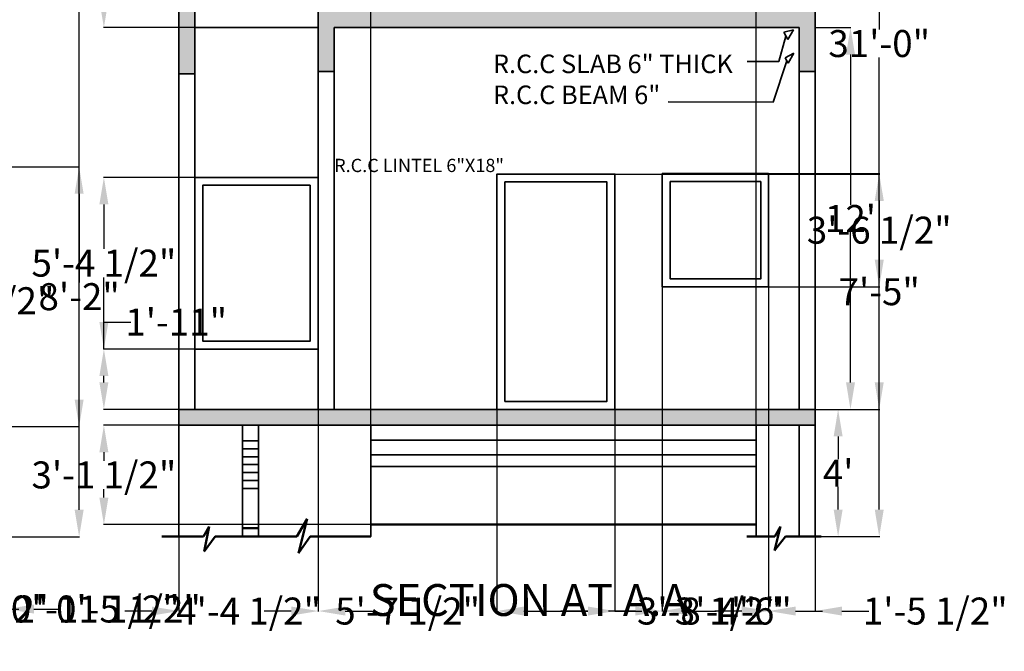
# Model space of a CAD drawing. Units: inches. Extents: x 21 to 3450, y 4 to 2137.
# Tile 7 of 14: x 2431 to 2802, y 1551 to 1790. Entities that reach past the tile are written whole.
import ezdxf

# ---------------------------------------------------------------- set-up
doc = ezdxf.new("R2010")
doc.units = ezdxf.units.IN
doc.header["$MEASUREMENT"] = 0
for name, color, linetype, lineweight in [('A-ANNO-DIMS', 2, 'Continuous', 18), ('A-ANNO-TEXT', 7, 'Continuous', 18), ('A-SECT', 7, 'Continuous', 35), ('A-SECT-PATT', 8, 'Continuous', 13), ('A-WALL', 7, 'Continuous', 50)]:
    doc.layers.add(name, color=color, linetype=linetype, lineweight=lineweight)
doc.styles.get("Standard").update_dxf_attribs({"font": 'arial.ttf'})
doc.dimstyles.get("Standard").update_dxf_attribs({"dimtxt": 10.18, "dimasz": 10.18, "dimexe": 0.18, "dimexo": 0.0625, "dimgap": 0.09, "dimtad": 0, "dimtih": 1, "dimtoh": 1, "dimdec": 0, "dimzin": 0, "dimdsep": 46, "dimlunit": 3, "dimtxsty": 'Standard', "dimcen": 0.09, "dimadec": 0, "dimazin": 0, "dimtfac": 1, "dimtdec": 0, "dimtofl": 0, "dimtmove": 0, "dimatfit": 3, "dimfxl": 1, "dimtolj": 1, "dimtzin": 0, "dimarcsym": 0})

# ---------------------------------------------------------------- blocks, each defined once
blk = doc.blocks.new('*D12')
at = {"layer": 'A-ANNO-DIMS', "color": 0, "lineweight": -2, "transparency": 16777216}
for p, q in [((2731.13, 1642.57), (2739.97, 1642.57)), ((2739.79, 1632.39), (2739.79, 1623.75)), ((2739.79, 1604.75), (2739.79, 1613.39)), ((2731.13, 1594.57), (2739.97, 1594.57))]:
    blk.add_line(p, q, dxfattribs=at)
at = {"layer": 'A-ANNO-DIMS', "color": 0, "transparency": 16777216}
for points in [[(2738.1, 1632.39), (2741.49, 1632.39), (2739.79, 1642.57)], [(2738.1, 1604.75), (2741.49, 1604.75), (2739.79, 1594.57)]]:
    blk.add_solid(points, dxfattribs=at)
at = {"layer": 'Defpoints', "color": 0, "transparency": 16777216}
for p in [(2731.07, 1642.57), (2739.79, 1642.57), (2731.07, 1594.57)]:
    blk.add_point(p, dxfattribs=at)
at = {"layer": 'A-ANNO-DIMS', "color": 0, "transparency": 16777216, "insert": (2739.79, 1618.57), "char_height": 10.18, "attachment_point": 5}
blk.add_mtext("\\A1;4'", dxfattribs=at)
blk = doc.blocks.new('*D13')
at = {"layer": 'A-ANNO-DIMS', "color": 0, "lineweight": -2, "transparency": 16777216}
for p, q in [((2731.13, 1786.57), (2744.63, 1786.57)), ((2744.45, 1776.39), (2744.45, 1719.77)), ((2744.45, 1652.75), (2744.45, 1709.37)), ((2731.19, 1642.57), (2744.63, 1642.57))]:
    blk.add_line(p, q, dxfattribs=at)
at = {"layer": 'A-ANNO-DIMS', "color": 0, "transparency": 16777216}
for points in [[(2742.76, 1776.39), (2746.15, 1776.39), (2744.45, 1786.57)], [(2742.76, 1652.75), (2746.15, 1652.75), (2744.45, 1642.57)]]:
    blk.add_solid(points, dxfattribs=at)
at = {"layer": 'Defpoints', "color": 0, "transparency": 16777216}
for p in [(2731.07, 1786.57), (2744.45, 1786.57), (2731.13, 1642.57)]:
    blk.add_point(p, dxfattribs=at)
at = {"layer": 'A-ANNO-DIMS', "color": 0, "transparency": 16777216, "insert": (2744.45, 1714.57), "char_height": 10.18, "attachment_point": 5}
blk.add_mtext("\\A1;12'", dxfattribs=at)
blk = doc.blocks.new('*D152')
at = {"layer": 'A-ANNO-DIMS', "color": 0, "lineweight": -2, "transparency": 16777216}
for p, q in [((2426.25, 2094.9), (2453.61, 2094.9)), ((2453.43, 2084.72), (2453.43, 1850.06)), ((2453.43, 1604.7), (2453.43, 1839.36)), ((2426.25, 1594.52), (2453.61, 1594.52))]:
    blk.add_line(p, q, dxfattribs=at)
at = {"layer": 'A-ANNO-DIMS', "color": 0, "transparency": 16777216}
for points in [[(2451.74, 2084.72), (2455.13, 2084.72), (2453.43, 2094.9)], [(2451.74, 1604.7), (2455.13, 1604.7), (2453.43, 1594.52)]]:
    blk.add_solid(points, dxfattribs=at)
at = {"layer": 'Defpoints', "color": 0, "transparency": 16777216}
for p in [(2426.18, 2094.9), (2453.43, 2094.9), (2426.18, 1594.52)]:
    blk.add_point(p, dxfattribs=at)
at = {"layer": 'A-ANNO-DIMS', "color": 0, "transparency": 16777216, "insert": (2453.43, 1844.71), "char_height": 10.18, "attachment_point": 5}
blk.add_mtext('\\A1;41\'-8 1/2"', dxfattribs=at)
blk = doc.blocks.new('*D165')
at = {"layer": 'A-ANNO-DIMS', "color": 0, "lineweight": -2, "transparency": 16777216}
for p, q in [((2374.7, 1636.02), (2374.7, 1567.09)), ((2384.8, 1636.02), (2384.8, 1567.09)), ((2364.52, 1567.27), (2354.34, 1567.27)), ((2394.98, 1567.27), (2405.16, 1567.27))]:
    blk.add_line(p, q, dxfattribs=at)
at = {"layer": 'A-ANNO-DIMS', "color": 0, "transparency": 16777216}
for points in [[(2364.52, 1568.97), (2364.52, 1565.57), (2374.7, 1567.27)], [(2394.98, 1568.97), (2394.98, 1565.57), (2384.8, 1567.27)]]:
    blk.add_solid(points, dxfattribs=at)
at = {"layer": 'Defpoints', "color": 0, "transparency": 16777216}
for p in [(2374.7, 1636.08), (2384.8, 1636.08), (2384.8, 1567.27)]:
    blk.add_point(p, dxfattribs=at)
at = {"layer": 'A-ANNO-DIMS', "color": 0, "transparency": 16777216, "insert": (2422.74, 1567.27), "char_height": 10.18, "attachment_point": 5}
blk.add_mtext('\\A1;0\'-10"', dxfattribs=at)
blk = doc.blocks.new('*D166')
at = {"layer": 'A-ANNO-DIMS', "color": 0, "lineweight": -2, "transparency": 16777216}
for p, q in [((2384.8, 1636.02), (2384.8, 1567.09)), ((2420.5, 1636.02), (2420.5, 1567.09)), ((2394.98, 1567.27), (2410.32, 1567.27)), ((2420.5, 1567.27), (2430.68, 1567.27))]:
    blk.add_line(p, q, dxfattribs=at)
at = {"layer": 'A-ANNO-DIMS', "color": 0, "transparency": 16777216}
for points in [[(2394.98, 1568.97), (2394.98, 1565.57), (2384.8, 1567.27)], [(2410.32, 1568.97), (2410.32, 1565.57), (2420.5, 1567.27)]]:
    blk.add_solid(points, dxfattribs=at)
at = {"layer": 'Defpoints', "color": 0, "transparency": 16777216}
for p in [(2384.8, 1636.08), (2420.5, 1636.08), (2420.5, 1567.27)]:
    blk.add_point(p, dxfattribs=at)
at = {"layer": 'A-ANNO-DIMS', "color": 0, "transparency": 16777216, "insert": (2460.2, 1567.27), "char_height": 10.18, "attachment_point": 5}
blk.add_mtext('\\A1;2\'-11 1/2"', dxfattribs=at)
blk = doc.blocks.new('*D167')
at = {"layer": 'A-ANNO-DIMS', "color": 0, "lineweight": -2, "transparency": 16777216}
for p, q in [((2420.5, 1636.02), (2420.5, 1567.09)), ((2426.18, 1636.02), (2426.18, 1567.09)), ((2410.32, 1567.27), (2400.14, 1567.27)), ((2436.36, 1567.27), (2446.54, 1567.27))]:
    blk.add_line(p, q, dxfattribs=at)
at = {"layer": 'A-ANNO-DIMS', "color": 0, "transparency": 16777216}
for points in [[(2410.32, 1568.97), (2410.32, 1565.57), (2420.5, 1567.27)], [(2436.36, 1568.97), (2436.36, 1565.57), (2426.18, 1567.27)]]:
    blk.add_solid(points, dxfattribs=at)
at = {"layer": 'Defpoints', "color": 0, "transparency": 16777216}
for p in [(2420.5, 1636.08), (2426.18, 1636.08), (2426.18, 1567.27)]:
    blk.add_point(p, dxfattribs=at)
at = {"layer": 'A-ANNO-DIMS', "color": 0, "transparency": 16777216, "insert": (2472.03, 1567.27), "char_height": 10.18, "attachment_point": 5}
blk.add_mtext('\\A1;0\'-5 1/2"', dxfattribs=at)
blk = doc.blocks.new('*D173')
at = {"layer": 'A-ANNO-DIMS', "color": 0, "lineweight": -2, "transparency": 16777216}
for p, q in [((2374.76, 1734.1), (2453.61, 1734.1)), ((2453.43, 1723.92), (2453.43, 1690.38)), ((2453.43, 1646.26), (2453.43, 1679.8)), ((2374.76, 1636.08), (2453.61, 1636.08))]:
    blk.add_line(p, q, dxfattribs=at)
at = {"layer": 'A-ANNO-DIMS', "color": 0, "transparency": 16777216}
for points in [[(2451.74, 1723.92), (2455.13, 1723.92), (2453.43, 1734.1)], [(2451.74, 1646.26), (2455.13, 1646.26), (2453.43, 1636.08)]]:
    blk.add_solid(points, dxfattribs=at)
at = {"layer": 'Defpoints', "color": 0, "transparency": 16777216}
for p in [(2374.7, 1734.1), (2453.43, 1734.1), (2374.7, 1636.08)]:
    blk.add_point(p, dxfattribs=at)
at = {"layer": 'A-ANNO-DIMS', "color": 0, "transparency": 16777216, "insert": (2453.43, 1685.09), "char_height": 10.18, "attachment_point": 5}
blk.add_mtext('\\A1;8\'-2"', dxfattribs=at)
blk = doc.blocks.new('*D178')
at = {"layer": 'A-ANNO-DIMS', "color": 0, "lineweight": -2, "transparency": 16777216}
for p, q in [((2731.13, 1966.57), (2755.48, 1966.57)), ((2755.3, 1956.39), (2755.3, 1785.86)), ((2755.3, 1604.75), (2755.3, 1775.27)), ((2731.13, 1594.57), (2755.48, 1594.57))]:
    blk.add_line(p, q, dxfattribs=at)
at = {"layer": 'A-ANNO-DIMS', "color": 0, "transparency": 16777216}
for points in [[(2753.61, 1956.39), (2757, 1956.39), (2755.3, 1966.57)], [(2753.61, 1604.75), (2757, 1604.75), (2755.3, 1594.57)]]:
    blk.add_solid(points, dxfattribs=at)
at = {"layer": 'Defpoints', "color": 0, "transparency": 16777216}
for p in [(2731.07, 1966.57), (2755.3, 1966.57), (2731.07, 1594.57)]:
    blk.add_point(p, dxfattribs=at)
at = {"layer": 'A-ANNO-DIMS', "color": 0, "transparency": 16777216, "insert": (2755.3, 1780.57), "char_height": 10.18, "attachment_point": 5}
blk.add_mtext('\\A1;31\'-0"', dxfattribs=at)
blk = doc.blocks.new('*D179')
at = {"layer": 'A-ANNO-DIMS', "color": 0, "lineweight": -2, "transparency": 16777216}
for p, q in [((2491.07, 1642.5), (2491.07, 1566.32)), ((2543.65, 1642.5), (2543.65, 1566.32)), ((2480.89, 1566.5), (2470.71, 1566.5)), ((2553.83, 1566.5), (2564.01, 1566.5))]:
    blk.add_line(p, q, dxfattribs=at)
at = {"layer": 'A-ANNO-DIMS', "color": 0, "transparency": 16777216}
for points in [[(2480.89, 1568.2), (2480.89, 1564.8), (2491.07, 1566.5)], [(2553.83, 1568.2), (2553.83, 1564.8), (2543.65, 1566.5)]]:
    blk.add_solid(points, dxfattribs=at)
at = {"layer": 'Defpoints', "color": 0, "transparency": 16777216}
for p in [(2491.07, 1642.57), (2543.65, 1642.57), (2543.65, 1566.5)]:
    blk.add_point(p, dxfattribs=at)
at = {"layer": 'A-ANNO-DIMS', "color": 0, "transparency": 16777216, "insert": (2517.36, 1566.5), "char_height": 10.18, "attachment_point": 5}
blk.add_mtext('\\A1;4\'-4 1/2"', dxfattribs=at)
blk = doc.blocks.new('*D180')
at = {"layer": 'A-ANNO-DIMS', "color": 0, "lineweight": -2, "transparency": 16777216}
for p, q in [((2543.65, 1642.5), (2543.65, 1566.32)), ((2611.07, 1642.5), (2611.07, 1566.32)), ((2533.47, 1566.5), (2523.29, 1566.5)), ((2621.25, 1566.5), (2631.43, 1566.5))]:
    blk.add_line(p, q, dxfattribs=at)
at = {"layer": 'A-ANNO-DIMS', "color": 0, "transparency": 16777216}
for points in [[(2533.47, 1568.2), (2533.47, 1564.8), (2543.65, 1566.5)], [(2621.25, 1568.2), (2621.25, 1564.8), (2611.07, 1566.5)]]:
    blk.add_solid(points, dxfattribs=at)
at = {"layer": 'Defpoints', "color": 0, "transparency": 16777216}
for p in [(2543.65, 1642.57), (2611.07, 1642.57), (2611.07, 1566.5)]:
    blk.add_point(p, dxfattribs=at)
at = {"layer": 'A-ANNO-DIMS', "color": 0, "transparency": 16777216, "insert": (2577.36, 1566.5), "char_height": 10.18, "attachment_point": 5}
blk.add_mtext('\\A1;5\'-7 1/2"', dxfattribs=at)
blk = doc.blocks.new('*D181')
at = {"layer": 'A-ANNO-DIMS', "color": 0, "lineweight": -2, "transparency": 16777216}
for p, q in [((2611.07, 1642.5), (2611.07, 1566.32)), ((2655.56, 1642.5), (2655.56, 1566.32)), ((2621.25, 1566.5), (2645.38, 1566.5)), ((2655.56, 1566.5), (2665.74, 1566.5))]:
    blk.add_line(p, q, dxfattribs=at)
at = {"layer": 'A-ANNO-DIMS', "color": 0, "transparency": 16777216}
for points in [[(2621.25, 1568.2), (2621.25, 1564.8), (2611.07, 1566.5)], [(2645.38, 1568.2), (2645.38, 1564.8), (2655.56, 1566.5)]]:
    blk.add_solid(points, dxfattribs=at)
at = {"layer": 'Defpoints', "color": 0, "transparency": 16777216}
for p in [(2611.07, 1642.57), (2655.56, 1642.57), (2655.56, 1566.5)]:
    blk.add_point(p, dxfattribs=at)
at = {"layer": 'A-ANNO-DIMS', "color": 0, "transparency": 16777216, "insert": (2691.22, 1566.5), "char_height": 10.18, "attachment_point": 5}
blk.add_mtext('\\A1;3\'-8 1/2"', dxfattribs=at)
blk = doc.blocks.new('*D182')
at = {"layer": 'A-ANNO-DIMS', "color": 0, "lineweight": -2, "transparency": 16777216}
for p, q in [((2673.46, 1688.74), (2673.46, 1566.32)), ((2655.56, 1642.5), (2655.56, 1566.32)), ((2645.38, 1566.5), (2635.2, 1566.5)), ((2683.64, 1566.5), (2693.82, 1566.5))]:
    blk.add_line(p, q, dxfattribs=at)
at = {"layer": 'A-ANNO-DIMS', "color": 0, "transparency": 16777216}
for points in [[(2645.38, 1568.2), (2645.38, 1564.8), (2655.56, 1566.5)], [(2683.64, 1568.2), (2683.64, 1564.8), (2673.46, 1566.5)]]:
    blk.add_solid(points, dxfattribs=at)
at = {"layer": 'Defpoints', "color": 0, "transparency": 16777216}
for p in [(2673.46, 1688.81), (2655.56, 1642.57), (2673.46, 1566.5)]:
    blk.add_point(p, dxfattribs=at)
at = {"layer": 'A-ANNO-DIMS', "color": 0, "transparency": 16777216, "insert": (2706.96, 1566.5), "char_height": 10.18, "attachment_point": 5}
blk.add_mtext('\\A1;1\'-6"', dxfattribs=at)
blk = doc.blocks.new('*D183')
at = {"layer": 'A-ANNO-DIMS', "color": 0, "lineweight": -2, "transparency": 16777216}
for p, q in [((2673.46, 1688.74), (2673.46, 1566.32)), ((2713.58, 1688.74), (2713.58, 1566.32)), ((2663.28, 1566.5), (2653.1, 1566.5)), ((2723.76, 1566.5), (2733.94, 1566.5))]:
    blk.add_line(p, q, dxfattribs=at)
at = {"layer": 'A-ANNO-DIMS', "color": 0, "transparency": 16777216}
for points in [[(2663.28, 1568.2), (2663.28, 1564.8), (2673.46, 1566.5)], [(2723.76, 1568.2), (2723.76, 1564.8), (2713.58, 1566.5)]]:
    blk.add_solid(points, dxfattribs=at)
at = {"layer": 'Defpoints', "color": 0, "transparency": 16777216}
for p in [(2673.46, 1688.81), (2713.58, 1688.81), (2713.58, 1566.5)]:
    blk.add_point(p, dxfattribs=at)
at = {"layer": 'A-ANNO-DIMS', "color": 0, "transparency": 16777216, "insert": (2693.52, 1566.5), "char_height": 10.18, "attachment_point": 5}
blk.add_mtext('\\A1;3\'-4"', dxfattribs=at)
blk = doc.blocks.new('*D184')
at = {"layer": 'A-ANNO-DIMS', "color": 0, "lineweight": -2, "transparency": 16777216}
for p, q in [((2713.58, 1688.74), (2713.58, 1566.32)), ((2731.07, 1642.5), (2731.07, 1566.32)), ((2703.4, 1566.5), (2693.22, 1566.5)), ((2741.25, 1566.5), (2751.43, 1566.5))]:
    blk.add_line(p, q, dxfattribs=at)
at = {"layer": 'A-ANNO-DIMS', "color": 0, "transparency": 16777216}
for points in [[(2703.4, 1568.2), (2703.4, 1564.8), (2713.58, 1566.5)], [(2741.25, 1568.2), (2741.25, 1564.8), (2731.07, 1566.5)]]:
    blk.add_solid(points, dxfattribs=at)
at = {"layer": 'Defpoints', "color": 0, "transparency": 16777216}
for p in [(2713.58, 1688.81), (2731.07, 1642.57), (2731.07, 1566.5)]:
    blk.add_point(p, dxfattribs=at)
at = {"layer": 'A-ANNO-DIMS', "color": 0, "transparency": 16777216, "insert": (2776.43, 1566.5), "char_height": 10.18, "attachment_point": 5}
blk.add_mtext('\\A1;1\'-5 1/2"', dxfattribs=at)
blk = doc.blocks.new('*D185')
at = {"layer": 'A-ANNO-DIMS', "color": 0, "lineweight": -2, "transparency": 16777216}
for p, q in [((2462.77, 1665.35), (2462.77, 1675.53)), ((2462.77, 1675.53), (2472.95, 1675.53)), ((2543.58, 1665.35), (2462.59, 1665.35)), ((2462.77, 1652.75), (2462.77, 1655.17)), ((2543.58, 1642.57), (2462.59, 1642.57))]:
    blk.add_line(p, q, dxfattribs=at)
at = {"layer": 'A-ANNO-DIMS', "color": 0, "transparency": 16777216}
for points in [[(2461.07, 1655.17), (2464.47, 1655.17), (2462.77, 1665.35)], [(2461.07, 1652.75), (2464.47, 1652.75), (2462.77, 1642.57)]]:
    blk.add_solid(points, dxfattribs=at)
at = {"layer": 'Defpoints', "color": 0, "transparency": 16777216}
for p in [(2462.77, 1665.35), (2543.65, 1665.35), (2543.65, 1642.57)]:
    blk.add_point(p, dxfattribs=at)
at = {"layer": 'A-ANNO-DIMS', "color": 0, "transparency": 16777216, "insert": (2490.05, 1675.53), "char_height": 10.18, "attachment_point": 5}
blk.add_mtext('\\A1;1\'-11"', dxfattribs=at)
blk = doc.blocks.new('*D186')
at = {"layer": 'A-ANNO-DIMS', "color": 0, "lineweight": -2, "transparency": 16777216}
for p, q in [((2543.58, 1730.1), (2462.59, 1730.1)), ((2462.77, 1719.92), (2462.77, 1703.08)), ((2462.77, 1675.53), (2462.77, 1692.37)), ((2543.58, 1665.35), (2462.59, 1665.35))]:
    blk.add_line(p, q, dxfattribs=at)
at = {"layer": 'A-ANNO-DIMS', "color": 0, "transparency": 16777216}
for points in [[(2461.07, 1719.92), (2464.47, 1719.92), (2462.77, 1730.1)], [(2461.07, 1675.53), (2464.47, 1675.53), (2462.77, 1665.35)]]:
    blk.add_solid(points, dxfattribs=at)
at = {"layer": 'Defpoints', "color": 0, "transparency": 16777216}
for p in [(2462.77, 1730.1), (2543.65, 1730.1), (2543.65, 1665.35)]:
    blk.add_point(p, dxfattribs=at)
at = {"layer": 'A-ANNO-DIMS', "color": 0, "transparency": 16777216, "insert": (2462.77, 1697.73), "char_height": 10.18, "attachment_point": 5}
blk.add_mtext('\\A1;5\'-4 1/2"', dxfattribs=at)
blk = doc.blocks.new('*D187')
at = {"layer": 'A-ANNO-DIMS', "color": 0, "lineweight": -2, "transparency": 16777216}
for p, q in [((2655.62, 1731.35), (2755.48, 1731.35)), ((2755.3, 1721.17), (2755.3, 1692.22)), ((2755.3, 1652.75), (2755.3, 1681.69)), ((2655.62, 1642.57), (2755.48, 1642.57))]:
    blk.add_line(p, q, dxfattribs=at)
at = {"layer": 'A-ANNO-DIMS', "color": 0, "transparency": 16777216}
for points in [[(2753.61, 1721.17), (2757, 1721.17), (2755.3, 1731.35)], [(2753.61, 1652.75), (2757, 1652.75), (2755.3, 1642.57)]]:
    blk.add_solid(points, dxfattribs=at)
at = {"layer": 'Defpoints', "color": 0, "transparency": 16777216}
for p in [(2655.56, 1731.35), (2755.3, 1731.35), (2655.56, 1642.57)]:
    blk.add_point(p, dxfattribs=at)
at = {"layer": 'A-ANNO-DIMS', "color": 0, "transparency": 16777216, "insert": (2755.3, 1686.96), "char_height": 10.18, "attachment_point": 5}
blk.add_mtext('\\A1;7\'-5"', dxfattribs=at)
blk = doc.blocks.new('*D188')
at = {"layer": 'A-ANNO-DIMS', "color": 0, "lineweight": -2, "transparency": 16777216}
for p, q in [((2713.65, 1731.52), (2755.48, 1731.52)), ((2755.3, 1721.34), (2755.3, 1715.52)), ((2755.3, 1698.99), (2755.3, 1704.8)), ((2713.65, 1688.81), (2755.48, 1688.81))]:
    blk.add_line(p, q, dxfattribs=at)
at = {"layer": 'A-ANNO-DIMS', "color": 0, "transparency": 16777216}
for points in [[(2753.61, 1721.34), (2757, 1721.34), (2755.3, 1731.52)], [(2753.61, 1698.99), (2757, 1698.99), (2755.3, 1688.81)]]:
    blk.add_solid(points, dxfattribs=at)
at = {"layer": 'Defpoints', "color": 0, "transparency": 16777216}
for p in [(2713.58, 1731.52), (2755.3, 1731.52), (2713.58, 1688.81)]:
    blk.add_point(p, dxfattribs=at)
at = {"layer": 'A-ANNO-DIMS', "color": 0, "transparency": 16777216, "insert": (2755.3, 1710.16), "char_height": 10.18, "attachment_point": 5}
blk.add_mtext('\\A1;3\'-6 1/2"', dxfattribs=at)
blk = doc.blocks.new('*D189')
at = {"layer": 'A-ANNO-DIMS', "color": 0, "lineweight": -2, "transparency": 16777216}
for p, q in [((2462.77, 1816.6), (2462.77, 1826.78)), ((2462.77, 1826.78), (2472.95, 1826.78)), ((2543.58, 1816.6), (2462.59, 1816.6)), ((2462.77, 1796.75), (2462.77, 1806.42)), ((2543.58, 1786.57), (2462.59, 1786.57))]:
    blk.add_line(p, q, dxfattribs=at)
at = {"layer": 'A-ANNO-DIMS', "color": 0, "transparency": 16777216}
for points in [[(2461.07, 1806.42), (2464.47, 1806.42), (2462.77, 1816.6)], [(2461.07, 1796.75), (2464.47, 1796.75), (2462.77, 1786.57)]]:
    blk.add_solid(points, dxfattribs=at)
at = {"layer": 'Defpoints', "color": 0, "transparency": 16777216}
for p in [(2462.77, 1816.6), (2543.65, 1816.6), (2543.65, 1786.57)]:
    blk.add_point(p, dxfattribs=at)
at = {"layer": 'A-ANNO-DIMS', "color": 0, "transparency": 16777216, "insert": (2486.66, 1826.78), "char_height": 10.18, "attachment_point": 5}
blk.add_mtext('\\A1;2\'-6"', dxfattribs=at)
blk = doc.blocks.new('*D193')
at = {"layer": 'A-ANNO-DIMS', "color": 0, "lineweight": -2, "transparency": 16777216}
for p, q in [((2563.42, 1636.57), (2462.59, 1636.57)), ((2462.77, 1626.39), (2462.77, 1623.2)), ((2462.77, 1609.31), (2462.77, 1612.49)), ((2563.42, 1599.13), (2462.59, 1599.13))]:
    blk.add_line(p, q, dxfattribs=at)
at = {"layer": 'A-ANNO-DIMS', "color": 0, "transparency": 16777216}
for points in [[(2461.07, 1626.39), (2464.47, 1626.39), (2462.77, 1636.57)], [(2461.07, 1609.31), (2464.47, 1609.31), (2462.77, 1599.13)]]:
    blk.add_solid(points, dxfattribs=at)
at = {"layer": 'Defpoints', "color": 0, "transparency": 16777216}
for p in [(2462.77, 1636.57), (2563.48, 1636.57), (2563.48, 1599.13)]:
    blk.add_point(p, dxfattribs=at)
at = {"layer": 'A-ANNO-DIMS', "color": 0, "transparency": 16777216, "insert": (2462.77, 1617.85), "char_height": 10.18, "attachment_point": 5}
blk.add_mtext('\\A1;3\'-1 1/2"', dxfattribs=at)
blk = doc.blocks.new('*D194')
at = {"layer": 'A-ANNO-DIMS', "color": 0, "lineweight": -2, "transparency": 16777216}
for p, q in [((2563.48, 1599.19), (2563.48, 2010.63)), ((2573.66, 2010.45), (2607.24, 2010.45)), ((2698.72, 2010.45), (2665.15, 2010.45)), ((2708.9, 1599.19), (2708.9, 2010.63))]:
    blk.add_line(p, q, dxfattribs=at)
at = {"layer": 'A-ANNO-DIMS', "color": 0, "transparency": 16777216}
for points in [[(2573.66, 2012.15), (2573.66, 2008.75), (2563.48, 2010.45)], [(2698.72, 2012.15), (2698.72, 2008.75), (2708.9, 2010.45)]]:
    blk.add_solid(points, dxfattribs=at)
at = {"layer": 'Defpoints', "color": 0, "transparency": 16777216}
for p in [(2708.9, 2010.45), (2563.48, 1599.13), (2708.9, 1599.13)]:
    blk.add_point(p, dxfattribs=at)
at = {"layer": 'A-ANNO-DIMS', "color": 0, "transparency": 16777216, "insert": (2636.19, 2010.45), "char_height": 10.18, "attachment_point": 5}
blk.add_mtext('\\A1;12\'-1 1/2"', dxfattribs=at)
blk = doc.blocks.new('*D195')
at = {"layer": 'A-ANNO-DIMS', "color": 0, "lineweight": -2, "transparency": 16777216}
for p, q in [((2329.47, 1683.55), (2329.65, 1683.55)), ((2329.56, 1683.46), (2329.56, 1683.64)), ((2358.76, 1683.55), (2348.58, 1683.55))]:
    blk.add_line(p, q, dxfattribs=at)
at = {"layer": 'A-ANNO-DIMS', "color": 0, "transparency": 16777216}
blk.add_solid([(2348.58, 1685.25), (2348.58, 1681.85), (2338.4, 1683.55)], dxfattribs=at)
at = {"layer": 'Defpoints', "color": 0, "transparency": 16777216}
for p in [(2320.73, 1683.55), (2338.4, 1683.55)]:
    blk.add_point(p, dxfattribs=at)
at = {"layer": 'A-ANNO-DIMS', "color": 0, "transparency": 16777216, "insert": (2400.44, 1683.55), "char_height": 10.18, "attachment_point": 5}
blk.add_mtext('\\A1;3X ∅1\'-5 1/2"', dxfattribs=at)

msp = doc.modelspace()

# ---------------------------------------------------------------- hatches: boundary and pattern name
at = {"layer": 'A-SECT-PATT'}
h = msp.add_hatch(color=256, dxfattribs=at)
h.dxf.hatch_style = 1
h.paths.add_polyline_path([(2731.07, 1792.57), (2725.07, 1792.57), (2543.65, 1792.57), (2543.65, 1770.05), (2549.65, 1770.05), (2549.65, 1786.57), (2725.07, 1786.57), (2725.07, 1770.05), (2731.07, 1770.05)])
h.paths.add_polyline_path([(2497.07, 1792.57), (2491.07, 1792.57), (2491.07, 1769.13), (2497.07, 1769.13)])
h = msp.add_hatch(color=256, dxfattribs=at)
h.dxf.hatch_style = 1
h.paths.add_polyline_path([(2725.07, 1642.57), (2491.07, 1642.57), (2491.07, 1636.57), (2725.07, 1636.57)])
h.paths.add_polyline_path([(2731.07, 1642.57), (2725.07, 1642.57), (2725.07, 1636.57), (2731.07, 1636.57)])

# ---------------------------------------------------------------- linework, layer by layer
at = {"layer": 'A-SECT'}
for p, q in [((2491.07, 1594.57), (2491.07, 1966.57)), ((2731.07, 1594.57), (2731.07, 1966.57)), ((2497.07, 1642.57), (2497.07, 1930.57)), ((2543.65, 1924.57), (2543.65, 1642.57)), ((2491.07, 1642.57), (2491.07, 1786.57)), ((2497.07, 1786.57), (2543.65, 1786.57)), ((2549.65, 1786.57), (2549.65, 1642.57)), ((2549.65, 1786.57), (2725.07, 1786.57)), ((2717.46, 1773.79), (2720.07, 1783.4)), ((2722.92, 1785.69), (2719.26, 1784.82)), ((2720.07, 1783.4), (2719.26, 1784.82)), ((2719.26, 1784.82), (2720.83, 1782.09)), ((2720.83, 1782.09), (2722.92, 1785.69)), ((2725.07, 1642.57), (2725.07, 1786.57)), ((2723.09, 1776.99), (2719.75, 1775.13)), ((2720.89, 1773.17), (2723.09, 1776.99)), ((2705.42, 1773.75), (2717.46, 1773.79)), ((2715.23, 1758.43), (2720.38, 1774.04)), ((2720.38, 1774.04), (2719.75, 1775.13)), ((2719.75, 1775.13), (2720.89, 1773.17)), ((2491.07, 1769.13), (2497.07, 1769.13)), ((2543.65, 1770.05), (2549.65, 1770.05)), ((2725.07, 1770.05), (2731.07, 1770.05)), ((2675.63, 1758.61), (2715.23, 1758.43)), ((2491.07, 1642.57), (2731.07, 1642.57)), ((2491.07, 1636.57), (2731.07, 1636.57)), ((2515.05, 1636.57), (2515.05, 1594.57)), ((2521.05, 1636.57), (2521.05, 1594.57)), ((2725.07, 1594.57), (2725.07, 1636.57)), ((2563.48, 1630.9), (2708.9, 1630.9)), ((2515.05, 1630.73), (2521.05, 1630.73)), ((2515.05, 1627.73), (2521.05, 1627.73)), ((2515.05, 1624.73), (2521.05, 1624.73)), ((2563.48, 1625.42), (2708.9, 1625.42)), ((2515.05, 1621.73), (2521.05, 1621.73)), ((2563.48, 1621.03), (2708.9, 1621.03)), ((2515.05, 1618.73), (2521.05, 1618.73)), ((2515.05, 1615.73), (2521.05, 1615.73)), ((2515.05, 1612.73), (2521.05, 1612.73))]:
    msp.add_line(p, q, dxfattribs=at)
for points in [[(2611.07, 1642.57), (2611.07, 1642.57), (2655.56, 1642.57), (2655.56, 1642.57), (2655.56, 1731.35), (2655.56, 1731.35), (2611.07, 1731.35), (2611.07, 1731.35)], [(2673.46, 1731.52), (2673.46, 1731.52), (2713.58, 1731.52), (2713.58, 1731.52), (2713.58, 1688.81), (2713.58, 1688.81), (2673.46, 1688.81), (2673.46, 1688.81)], [(2543.65, 1730.1), (2543.65, 1730.1), (2497.07, 1730.1), (2497.07, 1730.1), (2497.07, 1665.35), (2497.07, 1665.35), (2543.65, 1665.35), (2543.65, 1665.35)], [(2614.07, 1645.57), (2652.56, 1645.57), (2652.56, 1728.35), (2614.07, 1728.35)], [(2676.46, 1728.52), (2710.58, 1728.52), (2710.58, 1691.81), (2676.46, 1691.81)], [(2540.65, 1727.1), (2500.07, 1727.1), (2500.07, 1668.35), (2540.65, 1668.35)]]:
    msp.add_lwpolyline(points, close=True, dxfattribs=at)
for points in [[(2500.31, 1594.57), (2491.07, 1594.57), (2491.07, 1594.57), (2491.07, 1636.57), (2491.07, 1636.57), (2563.48, 1636.57), (2563.48, 1636.57), (2563.48, 1594.57), (2563.48, 1594.57), (2540.54, 1594.57)], [(2719.99, 1594.57), (2725.07, 1594.57), (2725.07, 1594.57), (2725.07, 1636.57), (2725.07, 1636.57), (2708.9, 1636.57), (2708.9, 1636.57), (2708.9, 1594.57), (2708.9, 1594.57), (2715.85, 1594.57)]]:
    msp.add_lwpolyline(points, dxfattribs=at)
at = {"layer": 'A-WALL'}
for p, q in [((2535.62, 1594.57), (2539.48, 1601.25)), ((2539.48, 1601.25), (2536.22, 1588.35)), ((2500.31, 1594.57), (2502.55, 1598.45)), ((2502.55, 1598.45), (2500.61, 1588.95)), ((2515.05, 1597.74), (2521.05, 1597.74)), ((2563.48, 1599.13), (2708.9, 1599.13)), ((2718.05, 1598.37), (2715.75, 1589.3)), ((2715.85, 1594.57), (2718.05, 1598.37)), ((2484.62, 1594.57), (2500.31, 1594.57)), ((2491.07, 1594.57), (2500.31, 1594.57)), ((2500.61, 1588.95), (2504.78, 1594.57)), ((2504.78, 1594.57), (2535.62, 1594.57)), ((2504.78, 1594.57), (2535.62, 1594.57)), ((2536.22, 1588.35), (2540.54, 1594.57)), ((2540.54, 1594.57), (2563.48, 1594.57)), ((2705.29, 1594.57), (2715.85, 1594.57)), ((2708.9, 1594.57), (2715.85, 1594.57)), ((2715.75, 1589.3), (2719.99, 1594.57)), ((2719.99, 1594.57), (2733.45, 1594.57)), ((2719.99, 1594.57), (2731.07, 1594.57))]:
    msp.add_line(p, q, dxfattribs=at)
msp.add_lwpolyline([(2535.62, 1594.57), (2504.78, 1594.57)], dxfattribs=at)

# ---------------------------------------------------------------- texts
at = {"layer": 'A-ANNO-TEXT', "attachment_point": 1}
for s, width, insert, char_height in [('R.C.C SLAB 6" THICK \\PR.C.C BEAM 6"', 108.6091, (2609.56, 1776.4), 7), ('R.C.C LINTEL 6"X18"', 267.3822, (2549.65, 1737.09), 5), ('SECTION AT A.A', 266.8546, (2563.06, 1576.67), 12)]:
    msp.add_mtext_dynamic_manual_height_columns(s, width=width, gutter_width=1, heights=[0], dxfattribs=dict(at, insert=insert, char_height=char_height))

# ---------------------------------------------------------------- dimensions: what is measured, and where the dimension line sits
at = {"layer": 'A-ANNO-DIMS'}
for base, p1, p2, override, picture, middle in [((2453.43, 2094.9), (2426.18, 1594.52), (2426.18, 2094.9), {"dimdec": 1, "dimlfac": 1, "dimrnd": 0, "dimzin": 1, "dimdsep": 46, "dimlunit": 4, "dimfrac": 2}, '*D152', (2453.43, 1844.71)), ((2755.3, 1966.57), (2731.07, 1594.57), (2731.07, 1966.57), {"dimdec": 1, "dimlfac": 1, "dimrnd": 0, "dimzin": 1, "dimdsep": 46, "dimlunit": 4, "dimfrac": 2}, '*D178', (2755.3, 1780.57)), ((2462.77, 1816.6), (2543.65, 1786.57), (2543.65, 1816.6), {"dimdec": 1, "dimlfac": 1, "dimrnd": 0, "dimzin": 1, "dimdsep": 46, "dimlunit": 4, "dimfrac": 2}, '*D189', (2486.66, 1826.78)), ((2744.45, 1786.57), (2731.13, 1642.57), (2731.07, 1786.57), {"dimclrd": 0, "dimclre": 0, "dimclrt": 0}, '*D13', (2744.45, 1714.57)), ((2453.43, 1734.1), (2374.7, 1636.08), (2374.7, 1734.1), {"dimdec": 1, "dimlfac": 1, "dimrnd": 0, "dimzin": 1, "dimdsep": 46, "dimlunit": 4, "dimfrac": 2}, '*D173', (2453.43, 1685.09)), ((2755.3, 1731.35), (2655.56, 1642.57), (2655.56, 1731.35), {"dimdec": 1, "dimlfac": 1, "dimrnd": 0, "dimzin": 1, "dimdsep": 46, "dimlunit": 4, "dimfrac": 2}, '*D187', (2755.3, 1686.96)), ((2755.3, 1731.52), (2713.58, 1688.81), (2713.58, 1731.52), {"dimdec": 1, "dimlfac": 1, "dimrnd": 0, "dimzin": 1, "dimdsep": 46, "dimlunit": 4, "dimfrac": 2}, '*D188', (2755.3, 1710.16)), ((2462.7694, 1730.0997), (2543.6453, 1665.353), (2543.6453, 1730.0997), {"dimdec": 1, "dimlfac": 1, "dimrnd": 0, "dimzin": 1, "dimdsep": 46, "dimlunit": 4, "dimfrac": 2}, '*D186', (2462.7694, 1697.7263)), ((2462.77, 1665.35), (2543.65, 1642.57), (2543.65, 1665.35), {"dimdec": 1, "dimlfac": 1, "dimrnd": 0, "dimzin": 1, "dimdsep": 46, "dimlunit": 4, "dimfrac": 2}, '*D185', (2490.05, 1675.53)), ((2739.79, 1642.57), (2731.07, 1594.57), (2731.07, 1642.57), {"dimclrd": 0, "dimclre": 0, "dimclrt": 0}, '*D12', (2739.79, 1618.57)), ((2462.77, 1636.57), (2563.48, 1599.13), (2563.48, 1636.57), {"dimdec": 1, "dimlfac": 1, "dimrnd": 0, "dimzin": 1, "dimdsep": 46, "dimlunit": 4, "dimfrac": 2}, '*D193', (2462.77, 1617.85))]:
    dim = msp.add_linear_dim(base=base, p1=p1, p2=p2, angle=90, dimstyle='Standard', override=override, dxfattribs=at)
    dim.commit()
    dim.dimension.update_dxf_attribs({"geometry": picture, "text_midpoint": middle})
for base, p1, p2, picture, middle in [((2708.9, 2010.45), (2563.48, 1599.13), (2708.9, 1599.13), '*D194', (2636.19, 2010.45)), ((2673.46, 1566.5), (2655.56, 1642.57), (2673.46, 1688.81), '*D182', (2706.96, 1566.5)), ((2713.58, 1566.5), (2673.46, 1688.81), (2713.58, 1688.81), '*D183', (2693.52, 1566.5)), ((2731.07, 1566.5), (2713.58, 1688.81), (2731.07, 1642.57), '*D184', (2776.43, 1566.5)), ((2543.65, 1566.5), (2491.07, 1642.57), (2543.65, 1642.57), '*D179', (2517.36, 1566.5)), ((2611.07, 1566.5), (2543.65, 1642.57), (2611.07, 1642.57), '*D180', (2577.36, 1566.5)), ((2655.56, 1566.5), (2611.07, 1642.57), (2655.56, 1642.57), '*D181', (2691.22, 1566.5)), ((2384.8, 1567.27), (2374.7, 1636.08), (2384.8, 1636.08), '*D165', (2422.74, 1567.27)), ((2420.5, 1567.27), (2384.8, 1636.08), (2420.5, 1636.08), '*D166', (2460.2, 1567.27)), ((2426.18, 1567.27), (2420.5, 1636.08), (2426.18, 1636.08), '*D167', (2472.03, 1567.27))]:
    dim = msp.add_linear_dim(base=base, p1=p1, p2=p2, dimstyle='Standard', override={"dimdec": 1, "dimlfac": 1, "dimrnd": 0, "dimzin": 1, "dimdsep": 46, "dimlunit": 4, "dimfrac": 2}, dxfattribs=at)
    dim.commit()
    dim.dimension.update_dxf_attribs({"geometry": picture, "text_midpoint": middle})
dim = msp.add_diameter_dim_2p(p1=(2320.73, 1683.55), p2=(2338.4, 1683.55), text='3X <>', dimstyle='Standard', override={"dimdec": 1, "dimlfac": 1, "dimrnd": 0, "dimzin": 1, "dimdsep": 46, "dimlunit": 4, "dimfrac": 2}, dxfattribs=at)
dim.commit()
dim.dimension.update_dxf_attribs({"geometry": '*D195', "text_midpoint": (2358.76, 1683.55), "dimtype": 163})

doc.saveas('drawing.dxf')
